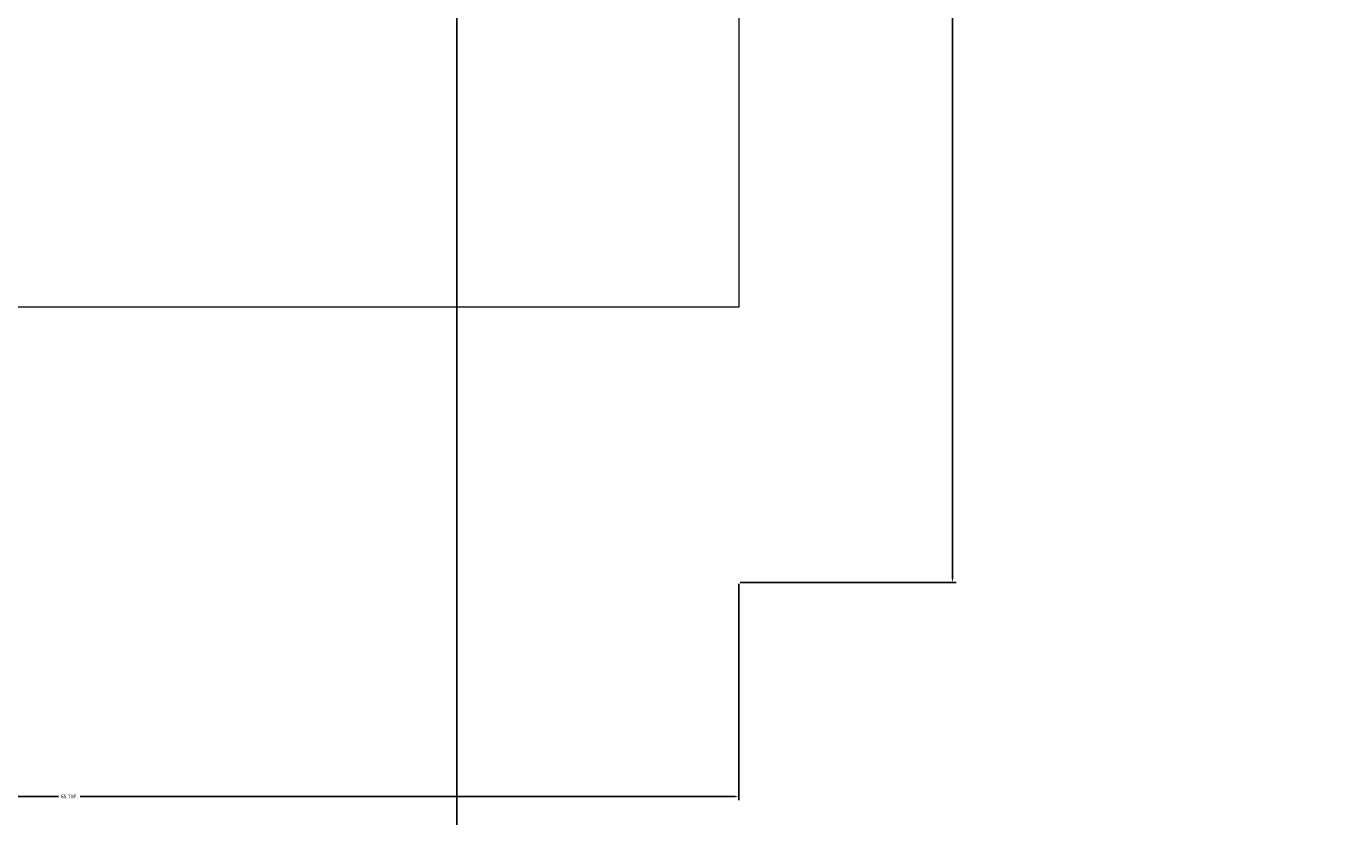
# Model space of a CAD drawing. Units: inches. Extents: x 1998 to 2588, y 1139 to 1977.
# Tile 68 of 134: x 2127 to 2192, y 1779 to 1817. Entities that reach past the tile are written whole.
import ezdxf

# ---------------------------------------------------------------- set-up
doc = ezdxf.new("R2010")
doc.units = ezdxf.units.IN
for name, color, linetype, lineweight in [('A-ANNO-DIMS', 2, 'Continuous', 18), ('DOOR', 52, 'Continuous', 25), ('FUR', 21, 'Continuous', 18)]:
    doc.layers.add(name, color=color, linetype=linetype, lineweight=lineweight)
doc.styles.get("Standard").update_dxf_attribs({"font": 'arial.ttf'})
doc.dimstyles.get("Standard").update_dxf_attribs({"dimtxt": 0.18, "dimasz": 0.18, "dimexe": 0.18, "dimexo": 0.0625, "dimgap": 0.09, "dimtad": 0, "dimtih": 1, "dimtoh": 1, "dimdec": 4, "dimzin": 0, "dimdsep": 46, "dimtxsty": 'Standard', "dimcen": 0.09, "dimadec": 0, "dimazin": 0, "dimtfac": 1, "dimtdec": 4, "dimtofl": 0, "dimtmove": 0, "dimatfit": 3, "dimfxl": 1, "dimtolj": 1, "dimtzin": 0, "dimarcsym": 0})

# ---------------------------------------------------------------- blocks, each defined once
blk = doc.blocks.new('*U2')
for p, q in [((0, 0), (0, -6)), ((40, 0), (40, -6))]:
    blk.add_line(p, q)
blk.add_lwpolyline([(0, 0), (0, 40), (1.75, 40), (1.75, 0)], close=True)
blk.add_arc((0, 0), 40, 0, 90)
blk = doc.blocks.new('BED-WITH-NIGHTSTANDS')
blk.add_lwpolyline([(0, 56), (65.221, 56), (65.221, 13.424), (0, 13.424)], close=True)
blk = doc.blocks.new('*D13')
at = {"layer": 'A-ANNO-DIMS', "color": 0, "lineweight": -2, "transparency": 16777216}
for p, q in [((2162.257, 1859.47), (2172.788, 1859.47)), ((2172.608, 1859.29), (2172.608, 1824.94)), ((2172.608, 1790.225), (2172.608, 1824.574)), ((2162.257, 1790.045), (2172.788, 1790.045))]:
    blk.add_line(p, q, dxfattribs=at)
at = {"layer": 'A-ANNO-DIMS', "color": 0, "transparency": 16777216}
for points in [[(2172.578, 1859.29), (2172.638, 1859.29), (2172.608, 1859.47)], [(2172.578, 1790.225), (2172.638, 1790.225), (2172.608, 1790.045)]]:
    blk.add_solid(points, dxfattribs=at)
at = {"layer": 'Defpoints', "color": 0, "transparency": 16777216}
for p in [(2162.194, 1859.47), (2172.608, 1859.47), (2162.194, 1790.045)]:
    blk.add_point(p, dxfattribs=at)
at = {"layer": 'A-ANNO-DIMS', "color": 0, "transparency": 16777216, "insert": (2172.608, 1824.757), "char_height": 0.18, "attachment_point": 5}
blk.add_mtext('\\A1;BED SET 69 TYP.', dxfattribs=at)
blk = doc.blocks.new('*D14')
at = {"layer": 'A-ANNO-DIMS', "color": 0, "lineweight": -2, "transparency": 16777216}
for p, q in [((2096.973, 1789.982), (2096.973, 1779.451)), ((2162.194, 1789.982), (2162.194, 1779.451)), ((2097.153, 1779.631), (2129.055, 1779.631)), ((2162.014, 1779.631), (2130.112, 1779.631))]:
    blk.add_line(p, q, dxfattribs=at)
at = {"layer": 'A-ANNO-DIMS', "color": 0, "transparency": 16777216}
for points in [[(2097.153, 1779.661), (2097.153, 1779.601), (2096.973, 1779.631)], [(2162.014, 1779.661), (2162.014, 1779.601), (2162.194, 1779.631)]]:
    blk.add_solid(points, dxfattribs=at)
at = {"layer": 'Defpoints', "color": 0, "transparency": 16777216}
for p in [(2096.973, 1790.045), (2162.194, 1790.045), (2162.194, 1779.631)]:
    blk.add_point(p, dxfattribs=at)
at = {"layer": 'A-ANNO-DIMS', "color": 0, "transparency": 16777216, "insert": (2129.584, 1779.631), "char_height": 0.18, "attachment_point": 5}
blk.add_mtext('\\A1;65 TYP.', dxfattribs=at)
blk = doc.blocks.new('*D37')
at = {"layer": 'A-ANNO-DIMS', "color": 0, "lineweight": -2, "transparency": 16777216}
for p, q in [((2148.455, 1612.795), (2148.455, 1977.362)), ((2148.635, 1977.182), (2172.73, 1977.182)), ((2197.27, 1977.182), (2173.175, 1977.182)), ((2197.45, 1612.795), (2197.45, 1977.362))]:
    blk.add_line(p, q, dxfattribs=at)
at = {"layer": 'A-ANNO-DIMS', "color": 0, "transparency": 16777216}
for points in [[(2148.635, 1977.212), (2148.635, 1977.152), (2148.455, 1977.182)], [(2197.27, 1977.212), (2197.27, 1977.152), (2197.45, 1977.182)]]:
    blk.add_solid(points, dxfattribs=at)
at = {"layer": 'Defpoints', "color": 0, "transparency": 16777216}
for p in [(2197.45, 1977.182), (2148.455, 1612.732), (2197.45, 1612.732)]:
    blk.add_point(p, dxfattribs=at)
at = {"layer": 'A-ANNO-DIMS', "color": 0, "transparency": 16777216, "insert": (2172.952, 1977.182), "char_height": 0.18, "attachment_point": 5}
blk.add_mtext('\\A1;49', dxfattribs=at)

msp = doc.modelspace()

# ---------------------------------------------------------------- block references
at = {"layer": 'DOOR', "xscale": -0.8354643497673233, "yscale": 0.8354643497673233, "zscale": 0.8354643497673233}
msp.add_blockref('*U2', (2221.7204, 1760.2452), dxfattribs=at)
at = {"layer": 'FUR'}
msp.add_blockref('BED-WITH-NIGHTSTANDS', (2096.973, 1790.045), dxfattribs=at)

# ---------------------------------------------------------------- dimensions: what is measured, and where the dimension line sits
at = {"layer": 'A-ANNO-DIMS'}
dim = msp.add_linear_dim(base=(2197.4499, 1977.1824), p1=(2148.4548, 1612.7324), p2=(2197.4499, 1612.7324), dimstyle='Standard', override={"dimdec": 0, "dimlfac": 1, "dimrnd": 0, "dimzin": 0, "dimdsep": 46, "dimlunit": 2}, dxfattribs=at)
dim.commit()
dim.dimension.update_dxf_attribs({"geometry": '*D37', "text_midpoint": (2172.9524, 1977.1824)})
dim = msp.add_linear_dim(base=(2172.6081, 1859.4697), p1=(2162.1944, 1790.0445), p2=(2162.1944, 1859.4697), angle=90, text='BED SET <> TYP.', dimstyle='Standard', override={"dimdec": 0, "dimlfac": 1, "dimrnd": 0, "dimzin": 0, "dimdsep": 46, "dimlunit": 2}, dxfattribs=at)
dim.commit()
dim.dimension.update_dxf_attribs({"geometry": '*D13', "text_midpoint": (2172.6081, 1824.7571)})
dim = msp.add_linear_dim(base=(2162.1944, 1779.6308), p1=(2096.9729, 1790.0445), p2=(2162.1944, 1790.0445), text='<> TYP.', dimstyle='Standard', override={"dimdec": 0, "dimlfac": 1, "dimrnd": 0, "dimzin": 0, "dimdsep": 46, "dimlunit": 2}, dxfattribs=at)
dim.commit()
dim.dimension.update_dxf_attribs({"geometry": '*D14', "text_midpoint": (2129.5836, 1779.6308)})

doc.saveas('drawing.dxf')
